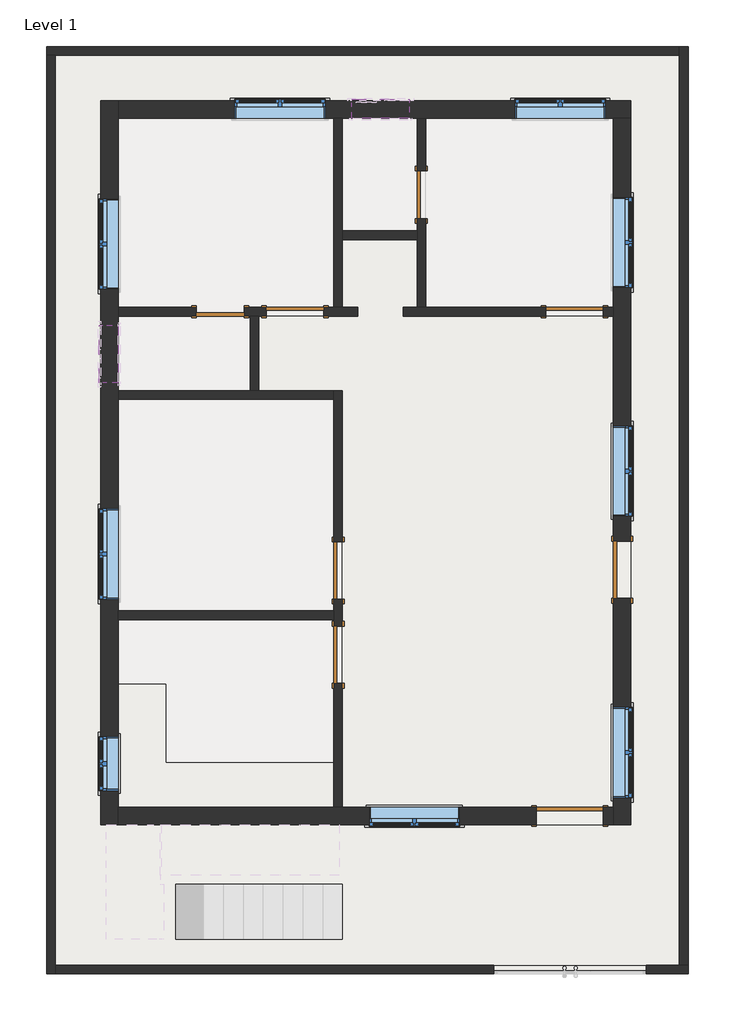
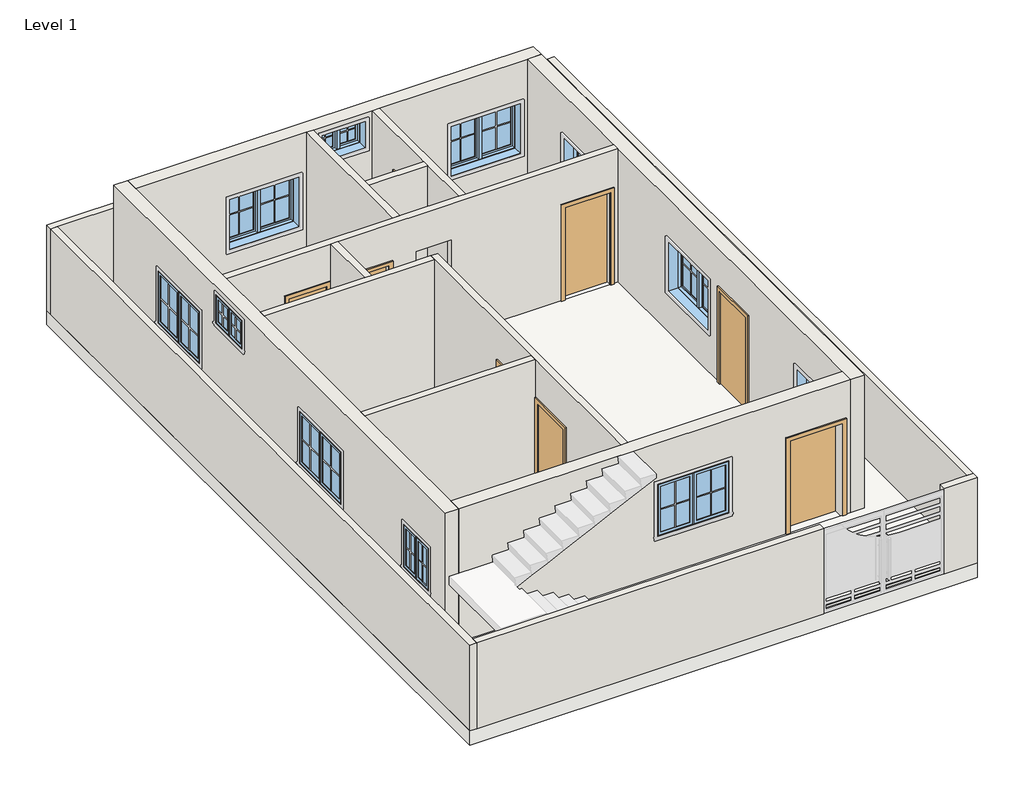
# One storey, part 1 of 2: 16 walls, 11 windows, 8 doors, 4 slabs.
"""IFC4 building model written with IfcOpenShell, lengths in millimetres."""

from ifc_helpers import new_model, si_unit, frame, origin, origin_with_axes, place, context, project, spatial, polyline, outline, extrude, faceted_brep, transform, mapped, element, save
from components import single_flush_3_6_472124c4, door_c78455d5, door_ad1ac78c, door_798417c2, door_6d3b6770, window_casement_double_3_v2_9f1923e6, window_6eb120d7, window_2333f571

model = new_model("IFC4")

# Units and contexts
model_context = context("Model", 3, world=origin())
ifc_project = project(units=[si_unit("LENGTHUNIT", "METRE", prefix="MILLI")], contexts=[model_context])

# Site, building, storey
site = spatial("IfcSite", under=ifc_project)
building = spatial("IfcBuilding", under=site)
storey = spatial("IfcBuildingStorey", under=building, Name="Level 1", Elevation=0.0)

# Doors
placement = place(None, origin())
single_flush_3_6_shape = single_flush_3_6_472124c4(model_context)
element("IfcDoor", 1, ObjectType="Single-Flush : 3'6", at=placement, inside=storey, context=model_context, shape_type="MappedRepresentation", body=[
    mapped(single_flush_3_6_shape, transform((-1353.6785282, -4927.3203663, 0.0), x_axis=(1.0, 0.0, 0.0), y_axis=(0.0, 1.0, 0.0), z_axis=(0.0, 0.0, 1.0))),
])
door_shape = door_c78455d5(model_context)
element("IfcDoor", 2, ObjectType="Single-Flush : 30\" x 80\"", at=placement, inside=storey, context=model_context, shape_type="MappedRepresentation", body=[
    mapped(door_shape, transform((-6936.6570389, 3131.9303819, 0.0), x_axis=(1.0, 0.0, 0.0), y_axis=(0.0, 1.0, 0.0), z_axis=(0.0, 0.0, 1.0))),
])
element("IfcDoor", 3, ObjectType="Single-Flush : 30\" x 80\"", at=placement, inside=storey, context=model_context, shape_type="MappedRepresentation", body=[
    mapped(door_shape, transform((-3724.1740631, 4999.2141951, 0.0), x_axis=(0.0, -1.0, 0.0), y_axis=(1.0, 0.0, 0.0), z_axis=(0.0, 0.0, 1.0))),
])
door_2_shape = door_ad1ac78c(model_context)
element("IfcDoor", 4, ObjectType="Single-Flush : 36\" x 80\"", at=placement, inside=storey, context=model_context, shape_type="MappedRepresentation", body=[
    mapped(door_2_shape, transform((-5742.8570389, 3131.9303819, 0.0), x_axis=(1.0, 0.0, 0.0), y_axis=(0.0, 1.0, 0.0), z_axis=(0.0, 0.0, 1.0))),
])
element("IfcDoor", 5, ObjectType="Single-Flush : 36\" x 80\"", at=placement, inside=storey, context=model_context, shape_type="MappedRepresentation", body=[
    mapped(door_2_shape, transform((-1277.4785282, 3131.9303819, 0.0), x_axis=(1.0, 0.0, 0.0), y_axis=(0.0, 1.0, 0.0), z_axis=(0.0, 0.0, 1.0))),
])
element("IfcDoor", 6, ObjectType="Single-Flush : 36\" x 80\"", at=placement, inside=storey, context=model_context, shape_type="MappedRepresentation", body=[
    mapped(door_2_shape, transform((-5055.0449828, -2348.5368209, 0.0), x_axis=(0.0, 1.0, 0.0), y_axis=(-1.0, 0.0, 0.0), z_axis=(0.0, 0.0, 1.0))),
])
door_3_shape = door_798417c2(model_context)
element("IfcDoor", 7, ObjectType="Single-Flush : 36\" x 80\"", at=placement, inside=storey, context=model_context, shape_type="MappedRepresentation", body=[
    mapped(door_3_shape, transform((-5055.0449828, -1002.3368209, 0.0), x_axis=(0.0, -1.0, 0.0), y_axis=(1.0, 0.0, 0.0), z_axis=(0.0, 0.0, 1.0))),
])
door_4_shape = door_6d3b6770(model_context)
element("IfcDoor", 8, ObjectType="Single-Flush : 36\" x 80\"", at=placement, inside=storey, context=model_context, shape_type="MappedRepresentation", body=[
    mapped(door_4_shape, transform((-515.4785282, -990.3203663, 0.0), x_axis=(0.0, -1.0, 0.0), y_axis=(1.0, 0.0, 0.0), z_axis=(0.0, 0.0, 1.0))),
])

# Slabs
element("IfcSlab", 9, at=placement, inside=storey, context=model_context, shape_type="SweptSolid", body=[
    extrude(outline(polyline([(398.9214718, 7227.9642844), (398.9214718, -7308.5703663), (-9573.0884077, -7308.5703663), (-9573.0884077, 7227.9642844), (398.9214718, 7227.9642844)]), holes=[polyline([(-8797.003757, -5067.0203663), (-375.7785282, -5067.0203663), (-375.7785282, 6451.8796337), (-8797.003757, 6451.8796337), (-8797.003757, -5067.0203663)])]), origin_with_axes(), (0.0, 0.0, 1.0), 50.8),
])
element("IfcSlab", 10, ObjectType="Generic - 12\"", at=placement, inside=storey, context=model_context, shape_type="SweptSolid", body=[
    extrude(outline(polyline([(538.6214718, 7367.6642844), (538.6214718, -7448.2703663), (-9712.7884077, -7448.2703663), (-9712.7884077, 7367.6642844), (538.6214718, 7367.6642844)])), frame((0.0, 0.0, -304.8), z_axis=(0.0, 0.0, 1.0), x_axis=(1.0, 0.0, 0.0)), (0.0, 0.0, 1.0), 304.8),
])
element("IfcSlab", 11, ObjectType="HALL FLOOR", at=placement, inside=storey, context=model_context, shape_type="SweptSolid", body=[
    extrude(outline(polyline([(-4985.1949828, -4787.6203663), (-4985.1949828, 1842.4631791), (-6320.7070389, 1842.4631791), (-6320.7070389, 3062.0803819), (-4744.7849815, 3062.0803819), (-4744.7849815, 3178.0086247), (-4985.1949828, 3178.0086247), (-4985.1949828, 4281.6641951), (-3765.6111695, 4281.6641951), (-3765.6111695, 3178.0086247), (-3997.4676553, 3178.0086247), (-3997.4676553, 3062.0803819), (-655.1785282, 3062.0803819), (-655.1785282, -4787.6203663), (-4985.1949828, -4787.6203663)])), origin_with_axes(), (0.0, 0.0, 1.0), 50.8),
])
element("IfcSlab", 12, ObjectType="KITCHEN BED", at=placement, inside=storey, context=model_context, shape_type="SweptSolid", body=[
    extrude(outline(polyline([(-7807.7884077, -2823.0618171), (-7807.7884077, -4077.7716275), (-5124.8949828, -4077.7716275), (-5124.8949828, -4839.7716275), (-7807.7884077, -4839.7716275), (-8569.7884077, -4839.7716275), (-8569.7884077, -2823.0618171), (-7807.7884077, -2823.0618171)])), frame((0.0, 0.0, 812.8), z_axis=(0.0, 0.0, 1.0), x_axis=(1.0, 0.0, 0.0)), (0.0, 0.0, 1.0), 101.6),
])

# Walls
element("IfcWall", 13, ObjectType="4.5\"", at=placement, inside=storey, context=model_context, shape_type="Brep", body=[
    faceted_brep([(-5124.8949828, -1459.5368209, 0.0), (-5124.8949828, -1648.7748314, 0.0), (-5124.8949828, -1788.4748314, 0.0), (-5124.8949828, -1891.3368209, 0.0), (-5124.8949828, -1891.3368209, 2032.0), (-5124.8949828, -2805.7368209, 2032.0), (-5124.8949828, -2805.7368209, 0.0), (-5124.8949828, -4787.6203663, 0.0), (-5124.8949828, -4787.6203663, 2895.6), (-5124.8949828, -1788.4748314, 2895.6), (-5124.8949828, -1648.7748314, 2895.6), (-5124.8949828, 1731.1760727, 2895.6), (-5124.8949828, 1870.8760727, 2895.6), (-5124.8949828, 1870.8760727, 0.0), (-5124.8949828, 1731.1760727, 0.0), (-5124.8949828, -545.1368209, 0.0), (-5124.8949828, -545.1368209, 2032.0), (-5124.8949828, -1459.5368209, 2032.0), (-4985.1949828, -1891.3368209, 2032.0), (-4985.1949828, -1891.3368209, 0.0), (-4985.1949828, -1459.5368209, 0.0), (-4985.1949828, -1459.5368209, 2032.0), (-4985.1949828, -545.1368209, 2032.0), (-4985.1949828, -545.1368209, 0.0), (-4985.1949828, 1870.8760727, 0.0), (-4985.1949828, 1870.8760727, 2895.6), (-4985.1949828, -4787.6203663, 2895.6), (-4985.1949828, -4787.6203663, 0.0), (-4985.1949828, -2805.7368209, 0.0), (-4985.1949828, -2805.7368209, 2032.0)], [[[0, 1, 2, 3, 4, 5, 6, 7, 8, 9, 10, 11, 12, 13, 14, 15, 16, 17]], [[18, 19, 20, 21, 22, 23, 24, 25, 26, 27, 28, 29]], [[28, 27, 7, 6]], [[20, 19, 3, 2, 1, 0]], [[15, 14, 13, 24, 23]], [[12, 11, 10, 9, 8, 26, 25]], [[8, 7, 27, 26]], [[21, 20, 0, 17]], [[22, 21, 17, 16]], [[23, 22, 16, 15]], [[4, 3, 19, 18]], [[5, 4, 18, 29]], [[6, 5, 29, 28]], [[13, 12, 25, 24]]]),
])
element("IfcWall", 14, ObjectType="4.5\"", at=placement, inside=storey, context=model_context, shape_type="SweptSolid", body=[
    extrude(outline(polyline([(-8569.7884077, -1648.7748314), (-5124.8949828, -1648.7748314), (-5124.8949828, -1788.4748314), (-8569.7884077, -1788.4748314), (-8569.7884077, -1648.7748314)])), origin_with_axes(), (0.0, 0.0, 1.0), 2895.6),
])
element("IfcWall", 15, ObjectType="4.5\"", at=placement, inside=storey, context=model_context, shape_type="Brep", body=[
    faceted_brep([(-5124.8949828, 1870.8760727, 0.0), (-6320.7070389, 1870.8760727, 0.0), (-6460.4070389, 1870.8760727, 0.0), (-8569.7884077, 1870.8760727, 0.0), (-8569.7884077, 1870.8760727, 2895.6), (-6460.4070389, 1870.8760727, 2895.6), (-6320.7070389, 1870.8760727, 2895.6), (-5124.8949828, 1870.8760727, 2895.6), (-5124.8949828, 1731.1760727, 0.0), (-5124.8949828, 1731.1760727, 2895.6), (-8569.7884077, 1731.1760727, 2895.6), (-8569.7884077, 1731.1760727, 0.0)], [[[0, 1, 2, 3, 4, 5, 6, 7]], [[8, 9, 10, 11]], [[3, 2, 1, 0, 8, 11]], [[7, 6, 5, 4, 10, 9]], [[4, 3, 11, 10]], [[0, 7, 9, 8]]]),
])
element("IfcWall", 16, ObjectType="4.5\"", at=placement, inside=storey, context=model_context, shape_type="SweptSolid", body=[
    extrude(outline(polyline([(-6460.4070389, 1870.8760727), (-6460.4070389, 3062.0803819), (-6320.7070389, 3062.0803819), (-6320.7070389, 1870.8760727), (-6460.4070389, 1870.8760727)])), origin_with_axes(), (0.0, 0.0, 1.0), 2895.6),
])
element("IfcWall", 17, ObjectType="4.5\"", at=placement, inside=storey, context=model_context, shape_type="Brep", body=[
    faceted_brep([(-6200.0570389, 3201.7803819, 0.0), (-6555.6570389, 3201.7803819, 0.0), (-6555.6570389, 3201.7803819, 2032.0), (-7317.6570389, 3201.7803819, 2032.0), (-7317.6570389, 3201.7803819, 0.0), (-8569.7884077, 3201.7803819, 0.0), (-8569.7884077, 3201.7803819, 2895.6), (-5124.8949828, 3201.7803819, 2895.6), (-4985.1949828, 3201.7803819, 2895.6), (-3794.0240631, 3201.7803819, 2895.6), (-3654.3240631, 3201.7803819, 2895.6), (-655.1785282, 3201.7803819, 2895.6), (-655.1785282, 3201.7803819, 0.0), (-820.2785282, 3201.7803819, 0.0), (-820.2785282, 3201.7803819, 2032.0), (-1734.6785282, 3201.7803819, 2032.0), (-1734.6785282, 3201.7803819, 0.0), (-3654.3240631, 3201.7803819, 0.0), (-3794.0240631, 3201.7803819, 0.0), (-4012.6375241, 3201.7803819, 0.0), (-4012.6375241, 3201.7803819, 2133.6), (-4744.7849815, 3201.7803819, 2133.6), (-4744.7849815, 3201.7803819, 0.0), (-4985.1949828, 3201.7803819, 0.0), (-5124.8949828, 3201.7803819, 0.0), (-5285.6570389, 3201.7803819, 0.0), (-5285.6570389, 3201.7803819, 2032.0), (-6200.0570389, 3201.7803819, 2032.0), (-6555.6570389, 3062.0803819, 2032.0), (-6555.6570389, 3062.0803819, 0.0), (-6460.4070389, 3062.0803819, 0.0), (-6320.7070389, 3062.0803819, 0.0), (-6200.0570389, 3062.0803819, 0.0), (-6200.0570389, 3062.0803819, 2032.0), (-5285.6570389, 3062.0803819, 2032.0), (-5285.6570389, 3062.0803819, 0.0), (-4744.7849815, 3062.0803819, 0.0), (-4744.7849815, 3062.0803819, 2133.6), (-4012.6375241, 3062.0803819, 2133.6), (-4012.6375241, 3062.0803819, 0.0), (-1734.6785282, 3062.0803819, 0.0), (-1734.6785282, 3062.0803819, 2032.0), (-820.2785282, 3062.0803819, 2032.0), (-820.2785282, 3062.0803819, 0.0), (-655.1785282, 3062.0803819, 0.0), (-655.1785282, 3062.0803819, 2895.6), (-6320.7070389, 3062.0803819, 2895.6), (-6460.4070389, 3062.0803819, 2895.6), (-8569.7884077, 3062.0803819, 2895.6), (-8569.7884077, 3062.0803819, 0.0), (-7317.6570389, 3062.0803819, 0.0), (-7317.6570389, 3062.0803819, 2032.0)], [[[0, 1, 2, 3, 4, 5, 6, 7, 8, 9, 10, 11, 12, 13, 14, 15, 16, 17, 18, 19, 20, 21, 22, 23, 24, 25, 26, 27]], [[28, 29, 30, 31, 32, 33, 34, 35, 36, 37, 38, 39, 40, 41, 42, 43, 44, 45, 46, 47, 48, 49, 50, 51]], [[36, 35, 25, 24, 23, 22]], [[40, 39, 19, 18, 17, 16]], [[44, 43, 13, 12]], [[50, 49, 5, 4]], [[32, 31, 30, 29, 1, 0]], [[11, 10, 9, 8, 7, 6, 48, 47, 46, 45]], [[6, 5, 49, 48]], [[12, 11, 45, 44]], [[20, 38, 37, 21]], [[38, 20, 19, 39]], [[21, 37, 36, 22]], [[26, 25, 35, 34]], [[27, 26, 34, 33]], [[0, 27, 33, 32]], [[14, 13, 43, 42]], [[15, 14, 42, 41]], [[16, 15, 41, 40]], [[2, 1, 29, 28]], [[3, 2, 28, 51]], [[4, 3, 51, 50]]]),
])
element("IfcWall", 18, ObjectType="4.5\"", at=placement, inside=storey, context=model_context, shape_type="Brep", body=[
    faceted_brep([(-5124.8949828, 6224.6642844, 0.0), (-5124.8949828, 3201.7803819, 0.0), (-5124.8949828, 3201.7803819, 2895.6), (-5124.8949828, 6224.6642844, 2895.6), (-4985.1949828, 6224.6642844, 0.0), (-4985.1949828, 6224.6642844, 2895.6), (-4985.1949828, 4421.3641951, 2895.6), (-4985.1949828, 4281.6641951, 2895.6), (-4985.1949828, 3201.7803819, 2895.6), (-4985.1949828, 3201.7803819, 0.0), (-4985.1949828, 4281.6641951, 0.0), (-4985.1949828, 4421.3641951, 0.0)], [[[0, 1, 2, 3]], [[4, 5, 6, 7, 8, 9, 10, 11]], [[1, 0, 4, 11, 10, 9]], [[3, 2, 8, 7, 6, 5]], [[0, 3, 5, 4]], [[2, 1, 9, 8]]]),
])
element("IfcWall", 19, ObjectType="4.5\"", at=placement, inside=storey, context=model_context, shape_type="Brep", body=[
    faceted_brep([(-3794.0240631, 4618.2141951, 2032.0), (-3794.0240631, 4618.2141951, 0.0), (-3794.0240631, 4421.3641951, 0.0), (-3794.0240631, 4281.6641951, 0.0), (-3794.0240631, 3201.7803819, 0.0), (-3794.0240631, 3201.7803819, 2895.6), (-3794.0240631, 4281.6641951, 2895.6), (-3794.0240631, 4421.3641951, 2895.6), (-3794.0240631, 6224.6642844, 2895.6), (-3794.0240631, 6224.6642844, 0.0), (-3794.0240631, 5380.2141951, 0.0), (-3794.0240631, 5380.2141951, 2032.0), (-3654.3240631, 3201.7803819, 0.0), (-3654.3240631, 4618.2141951, 0.0), (-3654.3240631, 4618.2141951, 2032.0), (-3654.3240631, 5380.2141951, 2032.0), (-3654.3240631, 5380.2141951, 0.0), (-3654.3240631, 6224.6642844, 0.0), (-3654.3240631, 6224.6642844, 2895.6), (-3654.3240631, 3201.7803819, 2895.6)], [[[0, 1, 2, 3, 4, 5, 6, 7, 8, 9, 10, 11]], [[12, 13, 14, 15, 16, 17, 18, 19]], [[10, 9, 17, 16]], [[4, 3, 2, 1, 13, 12]], [[8, 7, 6, 5, 19, 18]], [[9, 8, 18, 17]], [[14, 13, 1, 0]], [[15, 14, 0, 11]], [[16, 15, 11, 10]], [[5, 4, 12, 19]]]),
])
element("IfcWall", 20, ObjectType="4.5\"", at=placement, inside=storey, context=model_context, shape_type="SweptSolid", body=[
    extrude(outline(polyline([(-4985.1949828, 4421.3641951), (-3794.0240631, 4421.3641951), (-3794.0240631, 4281.6641951), (-4985.1949828, 4281.6641951), (-4985.1949828, 4421.3641951)])), origin_with_axes(), (0.0, 0.0, 1.0), 2895.6),
])
element("IfcWall", 21, ObjectType="4.5\"", at=placement, inside=storey, context=model_context, shape_type="Brep", body=[
    faceted_brep([(-9712.7884077, 7227.9642844, 0.0), (-9573.0884077, 7227.9642844, 0.0), (398.9214718, 7227.9642844, 0.0), (398.9214718, 7227.9642844, 1828.8), (-9573.0884077, 7227.9642844, 1828.8), (-9712.7884077, 7227.9642844, 1828.8), (-9712.7884077, 7367.6642844, 0.0), (-9712.7884077, 7367.6642844, 1828.8), (398.9214718, 7367.6642844, 1828.8), (398.9214718, 7367.6642844, 0.0)], [[[0, 1, 2, 3, 4, 5]], [[6, 7, 8, 9]], [[2, 1, 0, 6, 9]], [[5, 4, 3, 8, 7]], [[0, 5, 7, 6]], [[3, 2, 9, 8]]]),
])
element("IfcWall", 22, ObjectType="4.5\"", at=placement, inside=storey, context=model_context, shape_type="Brep", body=[
    faceted_brep([(-9573.0884077, -7448.2703663, 0.0), (-9573.0884077, -7308.5703663, 0.0), (-9573.0884077, 7227.9642844, 0.0), (-9573.0884077, 7227.9642844, 1828.8), (-9573.0884077, -7308.5703663, 1828.8), (-9573.0884077, -7448.2703663, 1828.8), (-9712.7884077, -7448.2703663, 0.0), (-9712.7884077, -7448.2703663, 1828.8), (-9712.7884077, 7227.9642844, 1828.8), (-9712.7884077, 7227.9642844, 0.0)], [[[0, 1, 2, 3, 4, 5]], [[6, 7, 8, 9]], [[2, 1, 0, 6, 9]], [[5, 4, 3, 8, 7]], [[0, 5, 7, 6]], [[3, 2, 9, 8]]]),
])
element("IfcWall", 23, ObjectType="4.5\"", at=placement, inside=storey, context=model_context, shape_type="Brep", body=[
    faceted_brep([(-9573.0884077, -7308.5703663, 0.0), (-9573.0884077, -7308.5703663, 1828.8), (-2567.7108489, -7308.5703663, 1828.8), (-2567.7108489, -7308.5703663, 0.0), (-9573.0884077, -7448.2703663, 1828.8), (-9573.0884077, -7448.2703663, 0.0), (-2567.7108489, -7448.2703663, 0.0), (-2567.7108489, -7448.2703663, 1828.8)], [[[0, 1, 2, 3]], [[4, 5, 6, 7]], [[5, 0, 3, 6]], [[1, 4, 7, 2]], [[1, 0, 5, 4]], [[3, 2, 7, 6]]]),
    faceted_brep([(538.6214718, -7308.5703663, 1828.8), (538.6214718, -7308.5703663, 0.0), (398.9214718, -7308.5703663, 0.0), (-128.4160269, -7308.5703663, 0.0), (-128.4160269, -7308.5703663, 1828.8), (398.9214718, -7308.5703663, 1828.8), (538.6214718, -7448.2703663, 0.0), (538.6214718, -7448.2703663, 1828.8), (-128.4160269, -7448.2703663, 1828.8), (-128.4160269, -7448.2703663, 0.0)], [[[0, 1, 2, 3, 4, 5]], [[6, 7, 8, 9]], [[1, 6, 9, 3, 2]], [[7, 0, 5, 4, 8]], [[1, 0, 7, 6]], [[4, 3, 9, 8]]]),
])
element("IfcWall", 24, ObjectType="4.5\"", at=placement, inside=storey, context=model_context, shape_type="Brep", body=[
    faceted_brep([(398.9214718, 7367.6642844, 0.0), (398.9214718, 7227.9642844, 0.0), (398.9214718, -7308.5703663, 0.0), (398.9214718, -7308.5703663, 1828.8), (398.9214718, 7227.9642844, 1828.8), (398.9214718, 7367.6642844, 1828.8), (538.6214718, 7367.6642844, 0.0), (538.6214718, 7367.6642844, 1828.8), (538.6214718, -7308.5703663, 1828.8), (538.6214718, -7308.5703663, 0.0)], [[[0, 1, 2, 3, 4, 5]], [[6, 7, 8, 9]], [[2, 1, 0, 6, 9]], [[5, 4, 3, 8, 7]], [[0, 5, 7, 6]], [[3, 2, 9, 8]]]),
])
element("IfcWall", 25, ObjectType="9\"", at=placement, inside=storey, context=model_context, shape_type="Brep", body=[
    faceted_brep([(-8849.1884077, 6504.0642844, 0.0), (-8849.1884077, -5067.0203663, 0.0), (-8849.1884077, -5067.0203663, 2895.6), (-8849.1884077, 6504.0642844, 2895.6), (-8849.1884077, -3657.3203663, 1828.8), (-8849.1884077, -4520.9203663, 1828.8), (-8849.1884077, -4520.9203663, 914.4), (-8849.1884077, -3657.3203663, 914.4), (-8849.1884077, 4935.3303819, 2032.0), (-8849.1884077, 3487.5303819, 2032.0), (-8849.1884077, 3487.5303819, 914.4), (-8849.1884077, 4935.3303819, 914.4), (-8849.1884077, -16.8248314, 2032.0), (-8849.1884077, -1464.6248314, 2032.0), (-8849.1884077, -1464.6248314, 914.4), (-8849.1884077, -16.8248314, 914.4), (-8849.1884077, 2910.9782273, 2743.2), (-8849.1884077, 1996.5782273, 2743.2), (-8849.1884077, 1996.5782273, 2133.6), (-8849.1884077, 2910.9782273, 2133.6), (-8569.7884077, 6504.0642844, 0.0), (-8569.7884077, 6504.0642844, 2895.6), (-8569.7884077, 6224.6642844, 2895.6), (-8569.7884077, 3201.7803819, 2895.6), (-8569.7884077, 3062.0803819, 2895.6), (-8569.7884077, 1870.8760727, 2895.6), (-8569.7884077, 1731.1760727, 2895.6), (-8569.7884077, -1648.7748314, 2895.6), (-8569.7884077, -1788.4748314, 2895.6), (-8569.7884077, -4787.6203663, 2895.6), (-8569.7884077, -5067.0203663, 2895.6), (-8569.7884077, -5067.0203663, 0.0), (-8569.7884077, -4787.6203663, 0.0), (-8569.7884077, -1788.4748314, 0.0), (-8569.7884077, -1648.7748314, 0.0), (-8569.7884077, 1731.1760727, 0.0), (-8569.7884077, 1870.8760727, 0.0), (-8569.7884077, 3062.0803819, 0.0), (-8569.7884077, 3201.7803819, 0.0), (-8569.7884077, 6224.6642844, 0.0), (-8569.7884077, -3657.3203663, 1828.8), (-8569.7884077, -3657.3203663, 914.4), (-8569.7884077, -4520.9203663, 914.4), (-8569.7884077, -4520.9203663, 1828.8), (-8569.7884077, 4935.3303819, 2032.0), (-8569.7884077, 4935.3303819, 914.4), (-8569.7884077, 3487.5303819, 914.4), (-8569.7884077, 3487.5303819, 2032.0), (-8569.7884077, -16.8248314, 2032.0), (-8569.7884077, -16.8248314, 914.4), (-8569.7884077, -1464.6248314, 914.4), (-8569.7884077, -1464.6248314, 2032.0), (-8569.7884077, 2910.9782273, 2743.2), (-8569.7884077, 2910.9782273, 2133.6), (-8569.7884077, 1996.5782273, 2133.6), (-8569.7884077, 1996.5782273, 2743.2)], [[[0, 1, 2, 3], [4, 5, 6, 7], [8, 9, 10, 11], [12, 13, 14, 15], [16, 17, 18, 19]], [[20, 21, 22, 23, 24, 25, 26, 27, 28, 29, 30, 31, 32, 33, 34, 35, 36, 37, 38, 39], [40, 41, 42, 43], [44, 45, 46, 47], [48, 49, 50, 51], [52, 53, 54, 55]], [[1, 0, 20, 39, 38, 37, 36, 35, 34, 33, 32, 31]], [[3, 2, 30, 29, 28, 27, 26, 25, 24, 23, 22, 21]], [[0, 3, 21, 20]], [[2, 1, 31, 30]], [[41, 40, 4, 7]], [[42, 41, 7, 6]], [[43, 42, 6, 5]], [[40, 43, 5, 4]], [[45, 44, 8, 11]], [[46, 45, 11, 10]], [[47, 46, 10, 9]], [[44, 47, 9, 8]], [[49, 48, 12, 15]], [[50, 49, 15, 14]], [[51, 50, 14, 13]], [[48, 51, 13, 12]], [[53, 52, 16, 19]], [[54, 53, 19, 18]], [[55, 54, 18, 17]], [[52, 55, 17, 16]]]),
])
element("IfcWall", 26, ObjectType="9\"", at=placement, inside=storey, context=model_context, shape_type="Brep", body=[
    faceted_brep([(-375.7785282, 6504.0642844, 0.0), (-8569.7884077, 6504.0642844, 0.0), (-8569.7884077, 6504.0642844, 2895.6), (-375.7785282, 6504.0642844, 2895.6), (-782.1785282, 6504.0642844, 2032.0), (-2229.9785282, 6504.0642844, 2032.0), (-2229.9785282, 6504.0642844, 914.4), (-782.1785282, 6504.0642844, 914.4), (-5258.2449828, 6504.0642844, 2032.0), (-6706.0449828, 6504.0642844, 2032.0), (-6706.0449828, 6504.0642844, 914.4), (-5258.2449828, 6504.0642844, 914.4), (-3919.7095229, 6504.0642844, 2743.2), (-4834.1095229, 6504.0642844, 2743.2), (-4834.1095229, 6504.0642844, 2133.6), (-3919.7095229, 6504.0642844, 2133.6), (-375.7785282, 6224.6642844, 0.0), (-375.7785282, 6224.6642844, 2895.6), (-655.1785282, 6224.6642844, 2895.6), (-3654.3240631, 6224.6642844, 2895.6), (-3794.0240631, 6224.6642844, 2895.6), (-4985.1949828, 6224.6642844, 2895.6), (-5124.8949828, 6224.6642844, 2895.6), (-8569.7884077, 6224.6642844, 2895.6), (-8569.7884077, 6224.6642844, 0.0), (-5124.8949828, 6224.6642844, 0.0), (-4985.1949828, 6224.6642844, 0.0), (-3794.0240631, 6224.6642844, 0.0), (-3654.3240631, 6224.6642844, 0.0), (-655.1785282, 6224.6642844, 0.0), (-782.1785282, 6224.6642844, 2032.0), (-782.1785282, 6224.6642844, 914.4), (-2229.9785282, 6224.6642844, 914.4), (-2229.9785282, 6224.6642844, 2032.0), (-5258.2449828, 6224.6642844, 2032.0), (-5258.2449828, 6224.6642844, 914.4), (-6706.0449828, 6224.6642844, 914.4), (-6706.0449828, 6224.6642844, 2032.0), (-3919.7095229, 6224.6642844, 2743.2), (-3919.7095229, 6224.6642844, 2133.6), (-4834.1095229, 6224.6642844, 2133.6), (-4834.1095229, 6224.6642844, 2743.2)], [[[0, 1, 2, 3], [4, 5, 6, 7], [8, 9, 10, 11], [12, 13, 14, 15]], [[16, 17, 18, 19, 20, 21, 22, 23, 24, 25, 26, 27, 28, 29], [30, 31, 32, 33], [34, 35, 36, 37], [38, 39, 40, 41]], [[1, 0, 16, 29, 28, 27, 26, 25, 24]], [[3, 2, 23, 22, 21, 20, 19, 18, 17]], [[2, 1, 24, 23]], [[0, 3, 17, 16]], [[31, 30, 4, 7]], [[32, 31, 7, 6]], [[33, 32, 6, 5]], [[30, 33, 5, 4]], [[35, 34, 8, 11]], [[36, 35, 11, 10]], [[37, 36, 10, 9]], [[34, 37, 9, 8]], [[39, 38, 12, 15]], [[40, 39, 15, 14]], [[41, 40, 14, 13]], [[38, 41, 13, 12]]]),
])
element("IfcWall", 27, ObjectType="9\"", at=placement, inside=storey, context=model_context, shape_type="Brep", body=[
    faceted_brep([(-655.1785282, -1447.5203663, 2032.0), (-655.1785282, -1447.5203663, 0.0), (-655.1785282, -4787.6203663, 0.0), (-655.1785282, -5067.0203663, 0.0), (-655.1785282, -5067.0203663, 2895.6), (-655.1785282, -4787.6203663, 2895.6), (-655.1785282, 3062.0803819, 2895.6), (-655.1785282, 3201.7803819, 2895.6), (-655.1785282, 6224.6642844, 2895.6), (-655.1785282, 6224.6642844, 0.0), (-655.1785282, 3201.7803819, 0.0), (-655.1785282, 3062.0803819, 0.0), (-655.1785282, -533.1203663, 0.0), (-655.1785282, -533.1203663, 2032.0), (-655.1785282, -4635.2203663, 2032.0), (-655.1785282, -4635.2203663, 914.4), (-655.1785282, -3187.4203663, 914.4), (-655.1785282, -3187.4203663, 2032.0), (-655.1785282, -139.4203663, 2032.0), (-655.1785282, -139.4203663, 914.4), (-655.1785282, 1308.3796337, 914.4), (-655.1785282, 1308.3796337, 2032.0), (-655.1785282, 3512.9303819, 2032.0), (-655.1785282, 3512.9303819, 914.4), (-655.1785282, 4960.7303819, 914.4), (-655.1785282, 4960.7303819, 2032.0), (-375.7785282, -5067.0203663, 0.0), (-375.7785282, -1447.5203663, 0.0), (-375.7785282, -1447.5203663, 2032.0), (-375.7785282, -533.1203663, 2032.0), (-375.7785282, -533.1203663, 0.0), (-375.7785282, 6224.6642844, 0.0), (-375.7785282, 6224.6642844, 2895.6), (-375.7785282, -5067.0203663, 2895.6), (-375.7785282, -4635.2203663, 2032.0), (-375.7785282, -3187.4203663, 2032.0), (-375.7785282, -3187.4203663, 914.4), (-375.7785282, -4635.2203663, 914.4), (-375.7785282, -139.4203663, 2032.0), (-375.7785282, 1308.3796337, 2032.0), (-375.7785282, 1308.3796337, 914.4), (-375.7785282, -139.4203663, 914.4), (-375.7785282, 3512.9303819, 2032.0), (-375.7785282, 4960.7303819, 2032.0), (-375.7785282, 4960.7303819, 914.4), (-375.7785282, 3512.9303819, 914.4)], [[[0, 1, 2, 3, 4, 5, 6, 7, 8, 9, 10, 11, 12, 13], [14, 15, 16, 17], [18, 19, 20, 21], [22, 23, 24, 25]], [[26, 27, 28, 29, 30, 31, 32, 33], [34, 35, 36, 37], [38, 39, 40, 41], [42, 43, 44, 45]], [[3, 2, 1, 27, 26]], [[12, 11, 10, 9, 31, 30]], [[8, 7, 6, 5, 4, 33, 32]], [[4, 3, 26, 33]], [[9, 8, 32, 31]], [[28, 27, 1, 0]], [[29, 28, 0, 13]], [[30, 29, 13, 12]], [[15, 14, 34, 37]], [[16, 15, 37, 36]], [[17, 16, 36, 35]], [[14, 17, 35, 34]], [[19, 18, 38, 41]], [[20, 19, 41, 40]], [[21, 20, 40, 39]], [[18, 21, 39, 38]], [[23, 22, 42, 45]], [[24, 23, 45, 44]], [[25, 24, 44, 43]], [[22, 25, 43, 42]]]),
])
element("IfcWall", 28, ObjectType="9\"", at=placement, inside=storey, context=model_context, shape_type="Brep", body=[
    faceted_brep([(-655.1785282, -4787.6203663, 0.0), (-820.2785282, -4787.6203663, 0.0), (-820.2785282, -4787.6203663, 2032.0), (-1887.0785282, -4787.6203663, 2032.0), (-1887.0785282, -4787.6203663, 0.0), (-4985.1949828, -4787.6203663, 0.0), (-5124.8949828, -4787.6203663, 0.0), (-8569.7884077, -4787.6203663, 0.0), (-8569.7884077, -4787.6203663, 2895.6), (-5124.8949828, -4787.6203663, 2895.6), (-4985.1949828, -4787.6203663, 2895.6), (-655.1785282, -4787.6203663, 2895.6), (-4559.7449828, -4787.6203663, 2032.0), (-4559.7449828, -4787.6203663, 914.4), (-3111.9449828, -4787.6203663, 914.4), (-3111.9449828, -4787.6203663, 2032.0), (-820.2785282, -5067.0203663, 2032.0), (-820.2785282, -5067.0203663, 0.0), (-655.1785282, -5067.0203663, 0.0), (-655.1785282, -5067.0203663, 2895.6), (-8569.7884077, -5067.0203663, 2895.6), (-8569.7884077, -5067.0203663, 0.0), (-1887.0785282, -5067.0203663, 0.0), (-1887.0785282, -5067.0203663, 2032.0), (-4559.7449828, -5067.0203663, 2032.0), (-3111.9449828, -5067.0203663, 2032.0), (-3111.9449828, -5067.0203663, 914.4), (-4559.7449828, -5067.0203663, 914.4)], [[[0, 1, 2, 3, 4, 5, 6, 7, 8, 9, 10, 11], [12, 13, 14, 15]], [[16, 17, 18, 19, 20, 21, 22, 23], [24, 25, 26, 27]], [[22, 21, 7, 6, 5, 4]], [[18, 17, 1, 0]], [[11, 10, 9, 8, 20, 19]], [[0, 11, 19, 18]], [[8, 7, 21, 20]], [[2, 1, 17, 16]], [[3, 2, 16, 23]], [[4, 3, 23, 22]], [[13, 12, 24, 27]], [[14, 13, 27, 26]], [[15, 14, 26, 25]], [[12, 15, 25, 24]]]),
])

# Windows
window_casement_double_3_v2_shape = window_casement_double_3_v2_9f1923e6(model_context)
element("IfcWindow", 29, ObjectType="Window-Casement-Double : 3'V2'", at=placement, inside=storey, context=model_context, shape_type="MappedRepresentation", body=[
    mapped(window_casement_double_3_v2_shape, transform((-8709.4884077, 2453.7782273, 1219.2), x_axis=(0.0, 1.0, 0.0), y_axis=(-1.0, 0.0, 0.0), z_axis=(0.0, 0.0, 1.0))),
])
element("IfcWindow", 30, ObjectType="Window-Casement-Double : 3'V2'", at=placement, inside=storey, context=model_context, shape_type="MappedRepresentation", body=[
    mapped(window_casement_double_3_v2_shape, transform((-4376.9095229, 6364.3642844, 1219.2), x_axis=(1.0, 0.0, 0.0), y_axis=(0.0, 1.0, 0.0), z_axis=(0.0, 0.0, 1.0))),
])
window_shape = window_6eb120d7(model_context)
element("IfcWindow", 31, ObjectType="Window-Casement-Double : 34\" x 36\"", at=placement, inside=storey, context=model_context, shape_type="MappedRepresentation", body=[
    mapped(window_shape, transform((-8709.4884077, -4089.1203663, 0.0), x_axis=(0.0, 1.0, 0.0), y_axis=(-1.0, 0.0, 0.0), z_axis=(0.0, 0.0, 1.0))),
])
window_2_shape = window_2333f571(model_context)
element("IfcWindow", 32, ObjectType="Window-Casement-Double : 57\" x 44\"", at=placement, inside=storey, context=model_context, shape_type="MappedRepresentation", body=[
    mapped(window_2_shape, transform((-515.4785282, -3911.3203663, 0.0), x_axis=(0.0, -1.0, 0.0), y_axis=(1.0, 0.0, 0.0), z_axis=(0.0, 0.0, 1.0))),
])
element("IfcWindow", 33, ObjectType="Window-Casement-Double : 57\" x 44\"", at=placement, inside=storey, context=model_context, shape_type="MappedRepresentation", body=[
    mapped(window_2_shape, transform((-515.4785282, 584.4796337, 0.0), x_axis=(0.0, -1.0, 0.0), y_axis=(1.0, 0.0, 0.0), z_axis=(0.0, 0.0, 1.0))),
])
element("IfcWindow", 34, ObjectType="Window-Casement-Double : 57\" x 44\"", at=placement, inside=storey, context=model_context, shape_type="MappedRepresentation", body=[
    mapped(window_2_shape, transform((-515.4785282, 4236.8303819, 0.0), x_axis=(0.0, -1.0, 0.0), y_axis=(1.0, 0.0, 0.0), z_axis=(0.0, 0.0, 1.0))),
])
element("IfcWindow", 35, ObjectType="Window-Casement-Double : 57\" x 44\"", at=placement, inside=storey, context=model_context, shape_type="MappedRepresentation", body=[
    mapped(window_2_shape, transform((-1506.0785282, 6364.3642844, 0.0), x_axis=(1.0, 0.0, 0.0), y_axis=(0.0, 1.0, 0.0), z_axis=(0.0, 0.0, 1.0))),
])
element("IfcWindow", 36, ObjectType="Window-Casement-Double : 57\" x 44\"", at=placement, inside=storey, context=model_context, shape_type="MappedRepresentation", body=[
    mapped(window_2_shape, transform((-5982.1449828, 6364.3642844, 0.0), x_axis=(1.0, 0.0, 0.0), y_axis=(0.0, 1.0, 0.0), z_axis=(0.0, 0.0, 1.0))),
])
element("IfcWindow", 37, ObjectType="Window-Casement-Double : 57\" x 44\"", at=placement, inside=storey, context=model_context, shape_type="MappedRepresentation", body=[
    mapped(window_2_shape, transform((-8709.4884077, 4211.4303819, 0.0), x_axis=(0.0, 1.0, 0.0), y_axis=(-1.0, 0.0, 0.0), z_axis=(0.0, 0.0, 1.0))),
])
element("IfcWindow", 38, ObjectType="Window-Casement-Double : 57\" x 44\"", at=placement, inside=storey, context=model_context, shape_type="MappedRepresentation", body=[
    mapped(window_2_shape, transform((-8709.4884077, -740.7248314, 0.0), x_axis=(0.0, 1.0, 0.0), y_axis=(-1.0, 0.0, 0.0), z_axis=(0.0, 0.0, 1.0))),
])
element("IfcWindow", 39, ObjectType="Window-Casement-Double : 57\" x 44\"", at=placement, inside=storey, context=model_context, shape_type="MappedRepresentation", body=[
    mapped(window_2_shape, transform((-3835.8449828, -4927.3203663, 0.0), x_axis=(-1.0, 0.0, 0.0), y_axis=(0.0, -1.0, 0.0), z_axis=(0.0, 0.0, 1.0))),
])

save(model, "model.ifc")

# Revit data of these elements
# Type "Single-Flush : 3'6"
#   Type Mark = "8"
#   Construction Type Id = "MDOOR"
#   Assembly Code = "C1020"
#   Analytic Construction = "Metal"
#   Thickness = 2"
#   Heat Transfer Coefficient (U) = 0.651978 BTU/(h·ft²·°F)
#   Height = 80"
#   Trim Projection Ext = 1"
#   Trim Projection Int = 1"
#   Trim Width = 3"
#   Width = 42"
#   Define Thermal Properties by = 1
#   Door Material = Door - Panel
#   Frame Material = Door - Frame
#   Visual Light Transmittance = 0
#   Solar Heat Gain Coefficient = 0
#   Function = (empty or 0)
#   Wall Closure = (empty or 0)
# Type "Single-Flush : 30\" x 80\""
#   Type Mark = "5"
#   Construction Type Id = "MDOOR"
#   Assembly Code = "C1020"
#   Analytic Construction = "Metal"
#   Thickness = 2"
#   Heat Transfer Coefficient (U) = 0.651978 BTU/(h·ft²·°F)
#   Height = 80"
#   Trim Projection Ext = 1"
#   Trim Projection Int = 1"
#   Trim Width = 3"
#   Width = 30"
#   Define Thermal Properties by = 1
#   Define Thermal Properties by = 1
#   Door Material = Door - Panel
#   Frame Material = Door - Frame
#   Visual Light Transmittance = 0
#   Solar Heat Gain Coefficient = 0
#   Function = (empty or 0)
#   Wall Closure = (empty or 0)
# Type "Single-Flush : 36\" x 80\""
#   Type Mark = "6"
#   Construction Type Id = "MDOOR"
#   Assembly Code = "C1020"
#   Analytic Construction = "Metal"
#   Thickness = 2"
#   Heat Transfer Coefficient (U) = 0.651978 BTU/(h·ft²·°F)
#   Height = 80"
#   Trim Projection Ext = 1"
#   Trim Projection Int = 1"
#   Trim Width = 3"
#   Width = 36"
#   Define Thermal Properties by = 1
#   Define Thermal Properties by = 1
#   Door Material = Door - Panel
#   Frame Material = Door - Frame
#   Visual Light Transmittance = 0
#   Solar Heat Gain Coefficient = 0
#   Function = (empty or 0)
#   Wall Closure = (empty or 0)
# Type
#   Assembly Code = "B1010"
#   Function = 0
# Type "Generic - 12\""
#   Assembly Code = "B1010"
#   Function = 0
#   Layers, outside or top first: 12" no material (function 1)
# Type "HALL FLOOR"
#   Assembly Code = "B1010"
#   Function = 0
#   Layers, outside or top first: 1" "HALL FLOORING" (function 1); 1" no material (function 1)
# Type "KITCHEN BED"
#   Assembly Code = "B1010"
#   Function = 0
#   Layers, outside or top first: 1" "KITCHEN BED" (function 1); 3" no material (function 1)
# Type "4.5\""
#   Assembly Code = "B2010"
#   Layers, outside or top first: 0.5" "INNER WALL" (function 1); 4.5" "BRICK MATERIAL" (function 1); 0.5" "INNER WALL" (function 1)
# Type "9\""
#   Assembly Code = "B2010"
#   Layers, outside or top first: 1" "OUTER WALL" (function 4); 9" "BRICK MATERIAL" (function 1); 1" "OUTER WALL" (function 1)
# Type "Window-Casement-Double : 3'V2'"
#   Type Mark = "18"
#   Fire Rating = "0.5h"
#   Assembly Code = "B2020100"
#   Analytic Construction = "Double glazing - domestic"
#   Frame Extension [instance default] = 0.25"
#   Window Inset [instance default] = 0"
#   Wall Thickness [instance default] = 6"
#   Interior Wall Closure [instance default] = 2.25"
#   Half Width = 18"
#   Visual Light Transmittance = 0.81
#   Thermal Resistance (R) = 1.8146 (h·ft²·°F)/BTU
#   Solar Heat Gain Coefficient = 0.76
#   Rough Width = 36.5"
#   Rough Height = 24.5"
#   Height = 24"
#   Heat Transfer Coefficient (U) = 0.5511 BTU/(h·ft²·°F)
#   Exterior Wall Closure [instance default] = 1.25"
#   Extension Jamb [instance default] = 2.25"
#   Default Sill Height = 36"
#   Width = 36"
#   Muntin Visibility = yes
#   Interior Trim Visibility [instance default] = yes
#   Exterior Trim Visibility [instance default] = yes
#   Extension Jamb Visibility [instance default] = yes
#   Interior Trim Material = Wood - Stained
#   Muntin Pattern = Muntin Pattern_2x2 : Muntin Pattern_2x2
#   Interior Trim = Trim-Window-Interior-Flat : Picture Frame
#   Interior Frame Material = Wood - Stained
#   Glass Panel Material = Glass
#   Exterior Trim Material = Clad - White
#   Exterior Trim = Trim-Window-Exterior-Flat : with Sill
#   Exterior Frame Material = Clad - White
#   Wall Closure = (empty or 0)
# Type "Window-Casement-Double : 34\" x 36\""
#   Type Mark = "14"
#   Fire Rating = "0.5h"
#   Assembly Code = "B2020100"
#   Analytic Construction = "Double glazing - domestic"
#   Frame Extension [instance default] = 0.25"
#   Window Inset [instance default] = 0"
#   Wall Thickness [instance default] = 6"
#   Interior Wall Closure [instance default] = 2.25"
#   Half Width = 17"
#   Visual Light Transmittance = 0.81
#   Thermal Resistance (R) = 1.8146 (h·ft²·°F)/BTU
#   Solar Heat Gain Coefficient = 0.76
#   Rough Width = 34.5"
#   Rough Height = 36.5"
#   Height = 36"
#   Heat Transfer Coefficient (U) = 0.5511 BTU/(h·ft²·°F)
#   Exterior Wall Closure [instance default] = 1.25"
#   Extension Jamb [instance default] = 2.25"
#   Default Sill Height = 36"
#   Width = 34"
#   Define Thermal Properties by = 0
#   Muntin Visibility = yes
#   Interior Trim Visibility [instance default] = yes
#   Exterior Trim Visibility [instance default] = yes
#   Extension Jamb Visibility [instance default] = yes
#   Interior Trim Material = Wood - Stained
#   Muntin Pattern = Muntin Pattern_2x2 : Muntin Pattern_2x2
#   Interior Trim = Trim-Window-Interior-Flat : Picture Frame
#   Interior Frame Material = Wood - Stained
#   Glass Panel Material = Glass
#   Exterior Trim Material = Clad - White
#   Exterior Trim = Trim-Window-Exterior-Flat : with Sill
#   Exterior Frame Material = Clad - White
#   Wall Closure = (empty or 0)
# Type "Window-Casement-Double : 57\" x 44\""
#   Type Mark = "17"
#   Fire Rating = "0.5h"
#   Assembly Code = "B2020100"
#   Analytic Construction = "Double glazing - domestic"
#   Frame Extension [instance default] = 0.25"
#   Window Inset [instance default] = 0"
#   Wall Thickness [instance default] = 6"
#   Interior Wall Closure [instance default] = 2.25"
#   Half Width = 28.5"
#   Visual Light Transmittance = 0.81
#   Thermal Resistance (R) = 1.8146 (h·ft²·°F)/BTU
#   Solar Heat Gain Coefficient = 0.76
#   Rough Width = 57.5"
#   Rough Height = 44.5"
#   Height = 44"
#   Heat Transfer Coefficient (U) = 0.5511 BTU/(h·ft²·°F)
#   Exterior Wall Closure [instance default] = 1.25"
#   Extension Jamb [instance default] = 2.25"
#   Default Sill Height = 36"
#   Width = 57"
#   Define Thermal Properties by = 0
#   Muntin Visibility = yes
#   Interior Trim Visibility [instance default] = yes
#   Exterior Trim Visibility [instance default] = yes
#   Extension Jamb Visibility [instance default] = yes
#   Interior Trim Material = Wood - Stained
#   Muntin Pattern = Muntin Pattern_2x2 : Muntin Pattern_2x2
#   Interior Trim = Trim-Window-Interior-Flat : Picture Frame
#   Interior Frame Material = Wood - Stained
#   Glass Panel Material = Glass
#   Exterior Trim Material = Clad - White
#   Exterior Trim = Trim-Window-Exterior-Flat : with Sill
#   Exterior Frame Material = Clad - White
#   Wall Closure = (empty or 0)
# Element 1 (IfcDoor, "Single-Flush : 3'6")
#   Phase Created = New Construction
#   Materials on its faces: "Door - Frame", "Door - Panel"
# Elements 2, 3 (IfcDoor, "Single-Flush : 30\" x 80\"")
#   Phase Created = New Construction
#   Materials on its faces: "Door - Frame", "Door - Panel"
# Elements 4, 5, 6, 7, 8 (IfcDoor, "Single-Flush : 36\" x 80\"")
#   Phase Created = New Construction
#   Materials on its faces: "Door - Frame", "Door - Panel"
# Element 9 (IfcSlab)
#   Height Offset From Level = 2"
#   Phase Created = New Construction
#   Materials on its faces: "Default Floor"
# Element 10 (IfcSlab, "Generic - 12\"")
#   Height Offset From Level = 0"
#   Phase Created = New Construction
#   Materials on its faces: "Default Floor"
# Element 11 (IfcSlab, "HALL FLOOR")
#   built-in parameter 1001955 = -1.5708 (stored number, unit not read)
#   Height Offset From Level = 2"
#   Phase Created = New Construction
#   Materials on its faces: "Default Floor", "HALL FLOORING"
# Element 12 (IfcSlab, "KITCHEN BED")
#   Height Offset From Level = 36"
#   Phase Created = New Construction
#   Materials on its faces: "Default Floor", "KITCHEN BED"
# Elements 13, 14, 15, 16, 17, 18, 19, 20 (IfcWall, "4.5\"")
#   Top Offset = -6"
#   Base Offset = 0"
#   wall height = 114"
#   Phase Created = New Construction
#   Base Constraint = Level 1
#   Top Constraint = Level 2
#   Materials on its faces: "Default Wall", "INNER WALL"
# Elements 21, 22, 24 (IfcWall, "4.5\"")
#   Top Offset = 0"
#   Base Offset = 0"
#   Unconnected Height = 72"
#   wall height = 72"
#   Phase Created = New Construction
#   Base Constraint = Level 1
#   Materials on its faces: "INNER WALL", "Default Wall"
# Element 23 (IfcWall, "4.5\"")
#   Top Offset = 0"
#   Base Offset = 0"
#   Unconnected Height = 72"
#   wall height = 72"
#   Phase Created = New Construction
#   Base Constraint = Level 1
#   Materials on its faces: "Default Wall", "INNER WALL"
# Elements 25, 26, 27, 28 (IfcWall, "9\"")
#   Top Offset = -6"
#   Base Offset = 0"
#   wall height = 114"
#   Phase Created = New Construction
#   Base Constraint = Level 1
#   Top Constraint = Level 2
#   Materials on its faces: "Default Wall", "OUTER WALL"
# Element 29 (IfcWindow, "Window-Casement-Double : 3'V2'")
#   Mark = "9"
#   Window Inset = 0"
#   Interior Wall Closure = 2.25"
#   Frame Extension = 0.25"
#   Exterior Wall Closure = 1.25"
#   Interior Trim Visibility = yes
#   Exterior Trim Visibility = yes
#   Phase Created = New Construction
#   Materials on its faces: "Wood - Stained", "Glass", "Clad - White"
# Element 30 (IfcWindow, "Window-Casement-Double : 3'V2'")
#   Mark = "10"
#   Window Inset = 0"
#   Interior Wall Closure = 2.25"
#   Frame Extension = 0.25"
#   Exterior Wall Closure = 1.25"
#   Interior Trim Visibility = yes
#   Exterior Trim Visibility = yes
#   Phase Created = New Construction
#   Materials on its faces: "Wood - Stained", "Glass", "Clad - White"
# Element 31 (IfcWindow, "Window-Casement-Double : 34\" x 36\"")
#   Mark = "1"
#   Window Inset = 0"
#   Interior Wall Closure = 2.25"
#   Frame Extension = 0.25"
#   Exterior Wall Closure = 1.25"
#   Interior Trim Visibility = yes
#   Exterior Trim Visibility = yes
#   Phase Created = New Construction
#   Materials on its faces: "Wood - Stained", "Glass", "Clad - White"
# Element 32 (IfcWindow, "Window-Casement-Double : 57\" x 44\"")
#   Mark = "2"
#   Window Inset = 0"
#   Interior Wall Closure = 2.25"
#   Frame Extension = 0.25"
#   Exterior Wall Closure = 1.25"
#   Interior Trim Visibility = yes
#   Exterior Trim Visibility = yes
#   Phase Created = New Construction
#   Materials on its faces: "Wood - Stained", "Glass", "Clad - White"
# Element 33 (IfcWindow, "Window-Casement-Double : 57\" x 44\"")
#   Mark = "3"
#   Window Inset = 0"
#   Interior Wall Closure = 2.25"
#   Frame Extension = 0.25"
#   Exterior Wall Closure = 1.25"
#   Interior Trim Visibility = yes
#   Exterior Trim Visibility = yes
#   Phase Created = New Construction
#   Materials on its faces: "Wood - Stained", "Glass", "Clad - White"
# Element 34 (IfcWindow, "Window-Casement-Double : 57\" x 44\"")
#   Mark = "4"
#   Window Inset = 0"
#   Interior Wall Closure = 2.25"
#   Frame Extension = 0.25"
#   Exterior Wall Closure = 1.25"
#   Interior Trim Visibility = yes
#   Exterior Trim Visibility = yes
#   Phase Created = New Construction
#   Materials on its faces: "Wood - Stained", "Glass", "Clad - White"
# Element 35 (IfcWindow, "Window-Casement-Double : 57\" x 44\"")
#   Mark = "5"
#   Window Inset = 0"
#   Interior Wall Closure = 2.25"
#   Frame Extension = 0.25"
#   Exterior Wall Closure = 1.25"
#   Interior Trim Visibility = yes
#   Exterior Trim Visibility = yes
#   Phase Created = New Construction
#   Materials on its faces: "Wood - Stained", "Glass", "Clad - White"
# Element 36 (IfcWindow, "Window-Casement-Double : 57\" x 44\"")
#   Mark = "6"
#   Window Inset = 0"
#   Interior Wall Closure = 2.25"
#   Frame Extension = 0.25"
#   Exterior Wall Closure = 1.25"
#   Interior Trim Visibility = yes
#   Exterior Trim Visibility = yes
#   Phase Created = New Construction
#   Materials on its faces: "Wood - Stained", "Glass", "Clad - White"
# Element 37 (IfcWindow, "Window-Casement-Double : 57\" x 44\"")
#   Mark = "7"
#   Window Inset = 0"
#   Interior Wall Closure = 2.25"
#   Frame Extension = 0.25"
#   Exterior Wall Closure = 1.25"
#   Interior Trim Visibility = yes
#   Exterior Trim Visibility = yes
#   Phase Created = New Construction
#   Materials on its faces: "Wood - Stained", "Glass", "Clad - White"
# Element 38 (IfcWindow, "Window-Casement-Double : 57\" x 44\"")
#   Mark = "8"
#   Window Inset = 0"
#   Interior Wall Closure = 2.25"
#   Frame Extension = 0.25"
#   Exterior Wall Closure = 1.25"
#   Interior Trim Visibility = yes
#   Exterior Trim Visibility = yes
#   Phase Created = New Construction
#   Materials on its faces: "Wood - Stained", "Glass", "Clad - White"
# Element 39 (IfcWindow, "Window-Casement-Double : 57\" x 44\"")
#   Mark = "11"
#   Window Inset = 0"
#   Interior Wall Closure = 2.25"
#   Frame Extension = 0.25"
#   Exterior Wall Closure = 1.25"
#   Interior Trim Visibility = yes
#   Exterior Trim Visibility = yes
#   Phase Created = New Construction
#   Materials on its faces: "Wood - Stained", "Glass", "Clad - White"
# Materials
#   "Door - Panel": class "Wood", colour RGB 210 159 95, transparency 0, Cost = 0
#   "Door - Frame": colour RGB 118 70 51, transparency 0, Cost = 0
#   "HALL FLOORING": class "Generic", colour RGB 240 240 231, transparency 0, Cost = 0
#   "KITCHEN BED": class "Generic", colour RGB 193 98 95, transparency 0, Cost = 0
#   "INNER WALL": class "Generic", colour RGB 112 107 80, transparency 0, Cost = 0
#   "BRICK MATERIAL": class "Generic", colour RGB 86 33 38, transparency 0, Cost = 0
#   "OUTER WALL": class "Generic", colour RGB 231 231 228, transparency 0, Cost = 0
#   "Wood - Stained": class "Wood", colour RGB 224 178 126, transparency 0, Cost = 0
#   "Glass": class "Glass", colour RGB 0 128 192, transparency 0.75, Description = "Soda Lime Glass", Cost = 0
#   "Clad - White": class "Wood", colour RGB 242 242 238, transparency 0, Cost = 0
#   "Default Floor": colour RGB 128 128 128, transparency 0, Cost = 0
#   "Default Wall": colour RGB 128 128 128, transparency 0, Cost = 0
